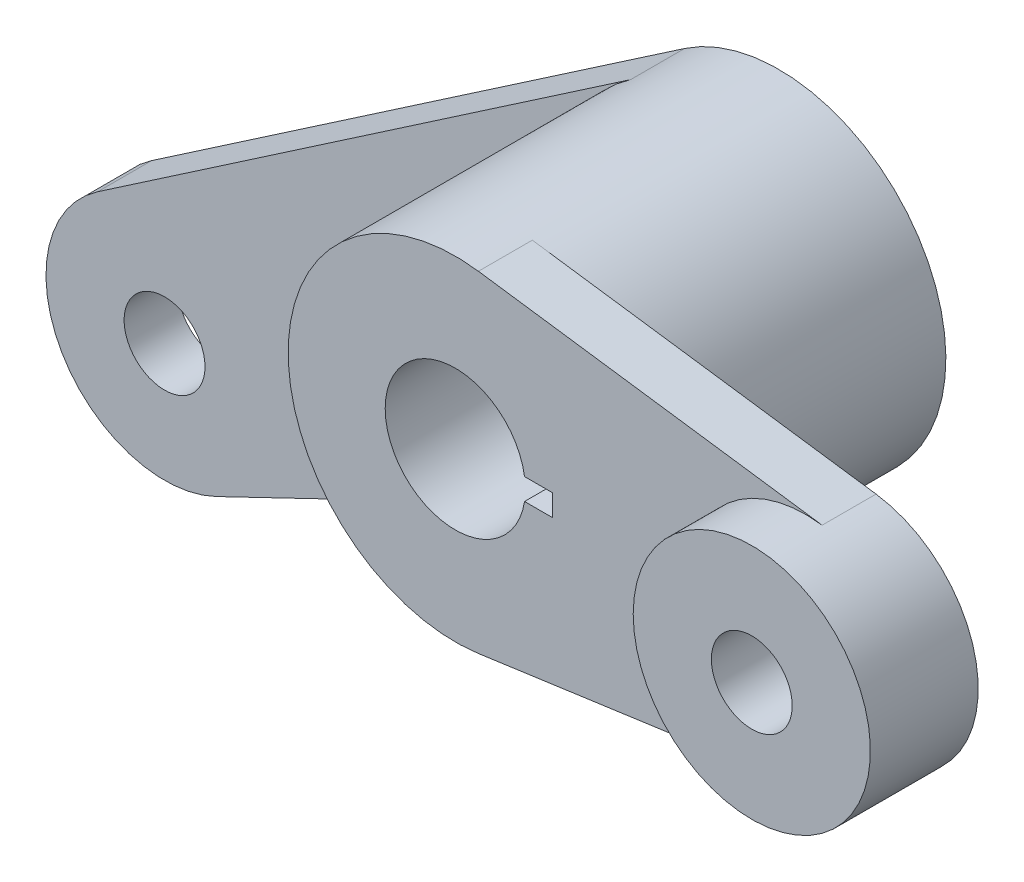
ISO-10303-21;
HEADER;
FILE_DESCRIPTION(('STEP AP214'),'2;1');
FILE_NAME('part.step','',(''),(''),'','','');
FILE_SCHEMA(('AUTOMOTIVE_DESIGN { 1 0 10303 214 1 1 1 1 }'));
ENDSEC;
DATA;
#1=APPLICATION_CONTEXT('core data for automotive mechanical design processes');
#2=APPLICATION_PROTOCOL_DEFINITION('international standard','automotive_design',2000,#1);
#3=PRODUCT_CONTEXT('',#1,'mechanical');
#4=PRODUCT('Part','Part','',(#3));
#5=PRODUCT_RELATED_PRODUCT_CATEGORY('part','',(#4));
#6=PRODUCT_DEFINITION_FORMATION('','',#4);
#7=PRODUCT_DEFINITION_CONTEXT('part definition',#1,'design');
#8=PRODUCT_DEFINITION('design','',#6,#7);
#9=PRODUCT_DEFINITION_SHAPE('','',#8);
#10=(LENGTH_UNIT() NAMED_UNIT(*) SI_UNIT(.MILLI.,.METRE.));
#11=(NAMED_UNIT(*) PLANE_ANGLE_UNIT() SI_UNIT($,.RADIAN.));
#12=(NAMED_UNIT(*) SI_UNIT($,.STERADIAN.) SOLID_ANGLE_UNIT());
#13=UNCERTAINTY_MEASURE_WITH_UNIT(LENGTH_MEASURE(1.E-05),#10,'distance_accuracy_value','');
#14=(GEOMETRIC_REPRESENTATION_CONTEXT(3) GLOBAL_UNCERTAINTY_ASSIGNED_CONTEXT((#13)) GLOBAL_UNIT_ASSIGNED_CONTEXT((#10,
#11,#12)) REPRESENTATION_CONTEXT('',''));
#15=CARTESIAN_POINT('',(0.,0.,0.));
#16=DIRECTION('',(0.,0.,1.));
#17=DIRECTION('',(1.,0.,0.));
#18=AXIS2_PLACEMENT_3D('',#15,#16,#17);
#19=CARTESIAN_POINT('',(65.,0.,-10.));
#20=DIRECTION('',(0.,0.,1.));
#21=DIRECTION('',(1.,0.,0.));
#22=AXIS2_PLACEMENT_3D('',#19,#20,#21);
#23=PLANE('',#22);
#24=CARTESIAN_POINT('',(65.,0.,-10.000012));
#25=DIRECTION('',(0.,0.,-1.));
#26=DIRECTION('',(-1.,0.,0.));
#27=AXIS2_PLACEMENT_3D('',#24,#25,#26);
#28=CIRCLE('',#27,7.5);
#29=CARTESIAN_POINT('',(57.5,0.,-10.000012));
#30=VERTEX_POINT('',#29);
#31=EDGE_CURVE('E198',#30,#30,#28,.T.);
#32=ORIENTED_EDGE('',*,*,#31,.F.);
#33=EDGE_LOOP('',(#32));
#34=FACE_BOUND('',#33,.T.);
#35=CARTESIAN_POINT('',(0.,0.,-10.));
#36=DIRECTION('',(0.,0.,-1.));
#37=DIRECTION('',(-1.,0.,0.));
#38=AXIS2_PLACEMENT_3D('',#35,#36,#37);
#39=CIRCLE('',#38,31.);
#40=CARTESIAN_POINT('',(4.29230769230769,30.7014021613762,-10.));
#41=VERTEX_POINT('',#40);
#42=CARTESIAN_POINT('',(4.29230769230769,-30.7014021613762,-10.));
#43=VERTEX_POINT('',#42);
#44=EDGE_CURVE('E193',#41,#43,#39,.T.);
#45=ORIENTED_EDGE('',*,*,#44,.F.);
#46=DIRECTION('',(-0.990367811657297,0.138461538461539,0.));
#47=VECTOR('',#46,1.);
#48=CARTESIAN_POINT('',(4.29230769230769,30.7014021613762,-10.));
#49=LINE('',#48,#47);
#50=CARTESIAN_POINT('',(68.0461538461538,21.7880918564605,-10.));
#51=VERTEX_POINT('',#50);
#52=EDGE_CURVE('E208',#51,#41,#49,.T.);
#53=ORIENTED_EDGE('',*,*,#52,.F.);
#54=CARTESIAN_POINT('',(65.,0.,-10.));
#55=DIRECTION('',(0.,0.,1.));
#56=DIRECTION('',(1.,0.,0.));
#57=AXIS2_PLACEMENT_3D('',#54,#55,#56);
#58=CIRCLE('',#57,22.);
#59=CARTESIAN_POINT('',(68.0461538461539,-21.7880918564605,-10.));
#60=VERTEX_POINT('',#59);
#61=EDGE_CURVE('E202',#60,#51,#58,.T.);
#62=ORIENTED_EDGE('',*,*,#61,.F.);
#63=DIRECTION('',(0.990367811657297,0.138461538461538,0.));
#64=VECTOR('',#63,1.);
#65=CARTESIAN_POINT('',(68.0461538461539,-21.7880918564605,-10.));
#66=LINE('',#65,#64);
#67=EDGE_CURVE('E215',#43,#60,#66,.T.);
#68=ORIENTED_EDGE('',*,*,#67,.F.);
#69=EDGE_LOOP('',(#45,#53,#62,#68));
#70=FACE_BOUND('',#69,.T.);
#71=ADVANCED_FACE('F39',(#34,#70),#23,.F.);
#72=CARTESIAN_POINT('',(65.,0.,-10.));
#73=DIRECTION('',(0.,0.,1.));
#74=DIRECTION('',(1.,0.,0.));
#75=AXIS2_PLACEMENT_3D('',#72,#73,#74);
#76=CYLINDRICAL_SURFACE('',#75,22.);
#77=DIRECTION('',(0.,0.,1.));
#78=VECTOR('',#77,1.);
#79=CARTESIAN_POINT('',(68.0461538461538,21.7880918564605,-10.));
#80=LINE('',#79,#78);
#81=CARTESIAN_POINT('',(68.0461538461538,21.7880918564605,0.));
#82=VERTEX_POINT('',#81);
#83=EDGE_CURVE('E214',#51,#82,#80,.T.);
#84=ORIENTED_EDGE('',*,*,#83,.T.);
#85=CARTESIAN_POINT('',(65.,0.,0.));
#86=DIRECTION('',(0.,0.,1.));
#87=DIRECTION('',(1.,0.,0.));
#88=AXIS2_PLACEMENT_3D('',#85,#86,#87);
#89=CIRCLE('',#88,22.);
#90=CARTESIAN_POINT('',(68.0461538461539,-21.7880918564605,0.));
#91=VERTEX_POINT('',#90);
#92=EDGE_CURVE('E223',#82,#91,#89,.T.);
#93=ORIENTED_EDGE('',*,*,#92,.T.);
#94=DIRECTION('',(0.,0.,1.));
#95=VECTOR('',#94,1.);
#96=CARTESIAN_POINT('',(68.0461538461539,-21.7880918564605,-10.));
#97=LINE('',#96,#95);
#98=EDGE_CURVE('E224',#60,#91,#97,.T.);
#99=ORIENTED_EDGE('',*,*,#98,.F.);
#100=ORIENTED_EDGE('',*,*,#61,.T.);
#101=EDGE_LOOP('',(#84,#93,#99,#100));
#102=FACE_BOUND('',#101,.T.);
#103=CARTESIAN_POINT('',(65.,0.,10.));
#104=DIRECTION('',(0.,0.,-1.));
#105=DIRECTION('',(-1.,0.,0.));
#106=AXIS2_PLACEMENT_3D('',#103,#104,#105);
#107=CIRCLE('',#106,22.);
#108=CARTESIAN_POINT('',(43.,0.,10.));
#109=VERTEX_POINT('',#108);
#110=EDGE_CURVE('E203',#109,#109,#107,.T.);
#111=ORIENTED_EDGE('',*,*,#110,.T.);
#112=EDGE_LOOP('',(#111));
#113=FACE_BOUND('',#112,.T.);
#114=ADVANCED_FACE('F41',(#102,#113),#76,.T.);
#115=CARTESIAN_POINT('',(68.0461538461539,-21.7880918564605,-10.));
#116=DIRECTION('',(0.138461538461538,-0.990367811657297,0.));
#117=DIRECTION('',(0.990367811657297,0.138461538461538,0.));
#118=AXIS2_PLACEMENT_3D('',#115,#116,#117);
#119=PLANE('',#118);
#120=DIRECTION('',(0.990367811657297,0.138461538461538,0.));
#121=VECTOR('',#120,1.);
#122=CARTESIAN_POINT('',(68.0461538461539,-21.7880918564605,0.));
#123=LINE('',#122,#121);
#124=CARTESIAN_POINT('',(4.29230769230769,-30.7014021613762,0.));
#125=VERTEX_POINT('',#124);
#126=EDGE_CURVE('E207',#125,#91,#123,.T.);
#127=ORIENTED_EDGE('',*,*,#126,.F.);
#128=DIRECTION('',(0.,0.,1.));
#129=VECTOR('',#128,1.);
#130=CARTESIAN_POINT('',(4.29230769230769,-30.7014021613762,-10.));
#131=LINE('',#130,#129);
#132=EDGE_CURVE('E228',#43,#125,#131,.T.);
#133=ORIENTED_EDGE('',*,*,#132,.F.);
#134=ORIENTED_EDGE('',*,*,#67,.T.);
#135=ORIENTED_EDGE('',*,*,#98,.T.);
#136=EDGE_LOOP('',(#127,#133,#134,#135));
#137=FACE_BOUND('',#136,.T.);
#138=ADVANCED_FACE('F259',(#137),#119,.T.);
#139=CARTESIAN_POINT('',(0.,0.,-10.));
#140=DIRECTION('',(0.,0.,1.));
#141=DIRECTION('',(1.,0.,0.));
#142=AXIS2_PLACEMENT_3D('',#139,#140,#141);
#143=CYLINDRICAL_SURFACE('',#142,31.);
#144=CARTESIAN_POINT('',(0.,0.,0.));
#145=DIRECTION('',(0.,0.,1.));
#146=DIRECTION('',(1.,0.,0.));
#147=AXIS2_PLACEMENT_3D('',#144,#145,#146);
#148=CIRCLE('',#147,31.);
#149=CARTESIAN_POINT('',(4.29230769230769,30.7014021613762,0.));
#150=VERTEX_POINT('',#149);
#151=EDGE_CURVE('E217',#150,#125,#148,.T.);
#152=ORIENTED_EDGE('',*,*,#151,.F.);
#153=DIRECTION('',(0.,0.,1.));
#154=VECTOR('',#153,1.);
#155=CARTESIAN_POINT('',(4.29230769230769,30.7014021613762,-10.));
#156=LINE('',#155,#154);
#157=EDGE_CURVE('E226',#41,#150,#156,.T.);
#158=ORIENTED_EDGE('',*,*,#157,.F.);
#159=ORIENTED_EDGE('',*,*,#44,.T.);
#160=ORIENTED_EDGE('',*,*,#132,.T.);
#161=EDGE_LOOP('',(#152,#158,#159,#160));
#162=FACE_BOUND('',#161,.T.);
#163=CARTESIAN_POINT('',(0.,0.,-50.));
#164=DIRECTION('',(0.,0.,-1.));
#165=DIRECTION('',(-1.,0.,0.));
#166=AXIS2_PLACEMENT_3D('',#163,#164,#165);
#167=CIRCLE('',#166,31.);
#168=CARTESIAN_POINT('',(13.442835709465,-27.9336744465946,-50.));
#169=VERTEX_POINT('',#168);
#170=CARTESIAN_POINT('',(-17.4698538370627,25.6086744465946,-50.));
#171=VERTEX_POINT('',#170);
#172=EDGE_CURVE('E53',#169,#171,#167,.T.);
#173=ORIENTED_EDGE('',*,*,#172,.F.);
#174=DIRECTION('',(0.,0.,1.));
#175=VECTOR('',#174,1.);
#176=CARTESIAN_POINT('',(13.442835709465,-27.9336744465946,-60.));
#177=LINE('',#176,#175);
#178=CARTESIAN_POINT('',(13.442835709465,-27.9336744465946,-60.));
#179=VERTEX_POINT('',#178);
#180=EDGE_CURVE('E182',#179,#169,#177,.T.);
#181=ORIENTED_EDGE('',*,*,#180,.F.);
#182=CARTESIAN_POINT('',(0.,0.,-60.));
#183=DIRECTION('',(0.,0.,1.));
#184=DIRECTION('',(1.,0.,0.));
#185=AXIS2_PLACEMENT_3D('',#182,#183,#184);
#186=CIRCLE('',#185,31.);
#187=CARTESIAN_POINT('',(-17.4698538370627,25.6086744465946,-60.));
#188=VERTEX_POINT('',#187);
#189=EDGE_CURVE('E159',#179,#188,#186,.T.);
#190=ORIENTED_EDGE('',*,*,#189,.T.);
#191=DIRECTION('',(0.,0.,1.));
#192=VECTOR('',#191,1.);
#193=CARTESIAN_POINT('',(-17.4698538370627,25.6086744465946,-60.));
#194=LINE('',#193,#192);
#195=EDGE_CURVE('E171',#188,#171,#194,.T.);
#196=ORIENTED_EDGE('',*,*,#195,.T.);
#197=EDGE_LOOP('',(#173,#181,#190,#196));
#198=FACE_BOUND('',#197,.T.);
#199=ADVANCED_FACE('F265',(#162,#198),#143,.T.);
#200=CARTESIAN_POINT('',(4.29230769230769,30.7014021613762,-10.));
#201=DIRECTION('',(0.138461538461539,0.990367811657297,0.));
#202=DIRECTION('',(-0.990367811657297,0.138461538461539,0.));
#203=AXIS2_PLACEMENT_3D('',#200,#201,#202);
#204=PLANE('',#203);
#205=DIRECTION('',(-0.990367811657297,0.138461538461539,0.));
#206=VECTOR('',#205,1.);
#207=CARTESIAN_POINT('',(4.29230769230769,30.7014021613762,0.));
#208=LINE('',#207,#206);
#209=EDGE_CURVE('E204',#82,#150,#208,.T.);
#210=ORIENTED_EDGE('',*,*,#209,.F.);
#211=ORIENTED_EDGE('',*,*,#83,.F.);
#212=ORIENTED_EDGE('',*,*,#52,.T.);
#213=ORIENTED_EDGE('',*,*,#157,.T.);
#214=EDGE_LOOP('',(#210,#211,#212,#213));
#215=FACE_BOUND('',#214,.T.);
#216=ADVANCED_FACE('F260',(#215),#204,.T.);
#217=CARTESIAN_POINT('',(65.,0.,0.));
#218=DIRECTION('',(0.,0.,1.));
#219=DIRECTION('',(1.,0.,0.));
#220=AXIS2_PLACEMENT_3D('',#217,#218,#219);
#221=PLANE('',#220);
#222=DIRECTION('',(0.,1.,0.));
#223=VECTOR('',#222,1.);
#224=CARTESIAN_POINT('',(18.,0.,0.));
#225=LINE('',#224,#223);
#226=CARTESIAN_POINT('',(18.,-2.,0.));
#227=VERTEX_POINT('',#226);
#228=CARTESIAN_POINT('',(18.,2.,0.));
#229=VERTEX_POINT('',#228);
#230=EDGE_CURVE('E11',#227,#229,#225,.T.);
#231=ORIENTED_EDGE('',*,*,#230,.F.);
#232=DIRECTION('',(1.,0.,0.));
#233=VECTOR('',#232,1.);
#234=CARTESIAN_POINT('',(65.,-1.99999999999997,0.));
#235=LINE('',#234,#233);
#236=CARTESIAN_POINT('',(12.8452325786651,-2.,0.));
#237=VERTEX_POINT('',#236);
#238=EDGE_CURVE('E131',#237,#227,#235,.T.);
#239=ORIENTED_EDGE('',*,*,#238,.F.);
#240=CARTESIAN_POINT('',(0.,0.,0.));
#241=DIRECTION('',(0.,0.,1.));
#242=DIRECTION('',(1.,0.,0.));
#243=AXIS2_PLACEMENT_3D('',#240,#241,#242);
#244=CIRCLE('',#243,13.);
#245=CARTESIAN_POINT('',(12.8452325786651,2.,0.));
#246=VERTEX_POINT('',#245);
#247=EDGE_CURVE('E181',#246,#237,#244,.T.);
#248=ORIENTED_EDGE('',*,*,#247,.F.);
#249=DIRECTION('',(-1.,0.,0.));
#250=VECTOR('',#249,1.);
#251=CARTESIAN_POINT('',(65.,1.99999999999998,0.));
#252=LINE('',#251,#250);
#253=EDGE_CURVE('E50',#229,#246,#252,.T.);
#254=ORIENTED_EDGE('',*,*,#253,.F.);
#255=EDGE_LOOP('',(#231,#239,#248,#254));
#256=FACE_BOUND('',#255,.T.);
#257=ORIENTED_EDGE('',*,*,#92,.F.);
#258=ORIENTED_EDGE('',*,*,#209,.T.);
#259=ORIENTED_EDGE('',*,*,#151,.T.);
#260=ORIENTED_EDGE('',*,*,#126,.T.);
#261=EDGE_LOOP('',(#257,#258,#259,#260));
#262=FACE_BOUND('',#261,.T.);
#263=ADVANCED_FACE('F255',(#256,#262),#221,.T.);
#264=CARTESIAN_POINT('',(65.,0.,10.));
#265=DIRECTION('',(0.,0.,-1.));
#266=DIRECTION('',(-1.,0.,0.));
#267=AXIS2_PLACEMENT_3D('',#264,#265,#266);
#268=PLANE('',#267);
#269=CARTESIAN_POINT('',(65.,0.,10.));
#270=DIRECTION('',(0.,0.,-1.));
#271=DIRECTION('',(-1.,0.,0.));
#272=AXIS2_PLACEMENT_3D('',#269,#270,#271);
#273=CIRCLE('',#272,7.5);
#274=CARTESIAN_POINT('',(57.5,0.,10.));
#275=VERTEX_POINT('',#274);
#276=EDGE_CURVE('E196',#275,#275,#273,.T.);
#277=ORIENTED_EDGE('',*,*,#276,.T.);
#278=EDGE_LOOP('',(#277));
#279=FACE_BOUND('',#278,.T.);
#280=ORIENTED_EDGE('',*,*,#110,.F.);
#281=EDGE_LOOP('',(#280));
#282=FACE_BOUND('',#281,.T.);
#283=ADVANCED_FACE('F252',(#279,#282),#268,.F.);
#284=CARTESIAN_POINT('',(65.,0.,10.));
#285=DIRECTION('',(0.,0.,-1.));
#286=DIRECTION('',(-1.,0.,0.));
#287=AXIS2_PLACEMENT_3D('',#284,#285,#286);
#288=CYLINDRICAL_SURFACE('',#287,7.5);
#289=ORIENTED_EDGE('',*,*,#276,.F.);
#290=EDGE_LOOP('',(#289));
#291=FACE_BOUND('',#290,.T.);
#292=ORIENTED_EDGE('',*,*,#31,.T.);
#293=EDGE_LOOP('',(#292));
#294=FACE_BOUND('',#293,.T.);
#295=ADVANCED_FACE('F286',(#291,#294),#288,.F.);
#296=CARTESIAN_POINT('',(0.,0.,-50.));
#297=DIRECTION('',(0.,0.,1.));
#298=DIRECTION('',(1.,0.,0.));
#299=AXIS2_PLACEMENT_3D('',#296,#297,#298);
#300=CYLINDRICAL_SURFACE('',#299,13.);
#301=DIRECTION('',(0.,0.,1.));
#302=VECTOR('',#301,1.);
#303=CARTESIAN_POINT('',(12.8452325786651,2.,-50.));
#304=LINE('',#303,#302);
#305=CARTESIAN_POINT('',(12.8452325786651,2.,-60.));
#306=VERTEX_POINT('',#305);
#307=EDGE_CURVE('E195',#306,#246,#304,.T.);
#308=ORIENTED_EDGE('',*,*,#307,.T.);
#309=ORIENTED_EDGE('',*,*,#247,.T.);
#310=DIRECTION('',(0.,0.,1.));
#311=VECTOR('',#310,1.);
#312=CARTESIAN_POINT('',(12.8452325786651,-2.,-50.));
#313=LINE('',#312,#311);
#314=CARTESIAN_POINT('',(12.8452325786651,-2.,-60.));
#315=VERTEX_POINT('',#314);
#316=EDGE_CURVE('E65',#315,#237,#313,.T.);
#317=ORIENTED_EDGE('',*,*,#316,.F.);
#318=CARTESIAN_POINT('',(0.,0.,-60.));
#319=DIRECTION('',(0.,0.,1.));
#320=DIRECTION('',(1.,0.,0.));
#321=AXIS2_PLACEMENT_3D('',#318,#319,#320);
#322=CIRCLE('',#321,13.);
#323=EDGE_CURVE('E149',#306,#315,#322,.T.);
#324=ORIENTED_EDGE('',*,*,#323,.F.);
#325=EDGE_LOOP('',(#308,#309,#317,#324));
#326=FACE_BOUND('',#325,.T.);
#327=ADVANCED_FACE('F292',(#326),#300,.F.);
#328=CARTESIAN_POINT('',(12.8452325786651,2.,-50.));
#329=DIRECTION('',(0.,-1.,0.));
#330=DIRECTION('',(0.,0.,-1.));
#331=AXIS2_PLACEMENT_3D('',#328,#329,#330);
#332=PLANE('',#331);
#333=DIRECTION('',(0.,0.,1.));
#334=VECTOR('',#333,1.);
#335=CARTESIAN_POINT('',(18.,2.,-50.));
#336=LINE('',#335,#334);
#337=CARTESIAN_POINT('',(18.,2.,-60.));
#338=VERTEX_POINT('',#337);
#339=EDGE_CURVE('E136',#338,#229,#336,.T.);
#340=ORIENTED_EDGE('',*,*,#339,.T.);
#341=ORIENTED_EDGE('',*,*,#253,.T.);
#342=ORIENTED_EDGE('',*,*,#307,.F.);
#343=DIRECTION('',(-1.,0.,0.));
#344=VECTOR('',#343,1.);
#345=CARTESIAN_POINT('',(18.,2.,-60.));
#346=LINE('',#345,#344);
#347=EDGE_CURVE('E145',#338,#306,#346,.T.);
#348=ORIENTED_EDGE('',*,*,#347,.F.);
#349=EDGE_LOOP('',(#340,#341,#342,#348));
#350=FACE_BOUND('',#349,.T.);
#351=ADVANCED_FACE('F296',(#350),#332,.T.);
#352=CARTESIAN_POINT('',(18.,-2.,-50.));
#353=DIRECTION('',(-1.,0.,0.));
#354=DIRECTION('',(0.,0.,1.));
#355=AXIS2_PLACEMENT_3D('',#352,#353,#354);
#356=PLANE('',#355);
#357=DIRECTION('',(0.,0.,1.));
#358=VECTOR('',#357,1.);
#359=CARTESIAN_POINT('',(18.,-2.,-50.));
#360=LINE('',#359,#358);
#361=CARTESIAN_POINT('',(18.,-2.,-60.));
#362=VERTEX_POINT('',#361);
#363=EDGE_CURVE('E127',#362,#227,#360,.T.);
#364=ORIENTED_EDGE('',*,*,#363,.T.);
#365=ORIENTED_EDGE('',*,*,#230,.T.);
#366=ORIENTED_EDGE('',*,*,#339,.F.);
#367=DIRECTION('',(0.,1.,0.));
#368=VECTOR('',#367,1.);
#369=CARTESIAN_POINT('',(18.,-2.,-60.));
#370=LINE('',#369,#368);
#371=EDGE_CURVE('E138',#362,#338,#370,.T.);
#372=ORIENTED_EDGE('',*,*,#371,.F.);
#373=EDGE_LOOP('',(#364,#365,#366,#372));
#374=FACE_BOUND('',#373,.T.);
#375=ADVANCED_FACE('F139',(#374),#356,.T.);
#376=CARTESIAN_POINT('',(12.8452325786651,-2.,-50.));
#377=DIRECTION('',(0.,1.,0.));
#378=DIRECTION('',(-1.,0.,0.));
#379=AXIS2_PLACEMENT_3D('',#376,#377,#378);
#380=PLANE('',#379);
#381=ORIENTED_EDGE('',*,*,#316,.T.);
#382=ORIENTED_EDGE('',*,*,#238,.T.);
#383=ORIENTED_EDGE('',*,*,#363,.F.);
#384=DIRECTION('',(1.,0.,0.));
#385=VECTOR('',#384,1.);
#386=CARTESIAN_POINT('',(12.8452325786651,-2.,-60.));
#387=LINE('',#386,#385);
#388=EDGE_CURVE('E128',#315,#362,#387,.T.);
#389=ORIENTED_EDGE('',*,*,#388,.F.);
#390=EDGE_LOOP('',(#381,#382,#383,#389));
#391=FACE_BOUND('',#390,.T.);
#392=ADVANCED_FACE('F126',(#391),#380,.T.);
#393=CARTESIAN_POINT('',(-94.3829714990283,-79.8238979943576,-60.));
#394=DIRECTION('',(0.433639861595647,-0.901086272470793,0.));
#395=DIRECTION('',(0.901086272470793,0.433639861595647,0.));
#396=AXIS2_PLACEMENT_3D('',#393,#394,#395);
#397=PLANE('',#396);
#398=DIRECTION('',(0.901086272470793,0.433639861595647,0.));
#399=VECTOR('',#398,1.);
#400=CARTESIAN_POINT('',(-94.3829714990283,-79.8238979943576,-50.));
#401=LINE('',#400,#399);
#402=CARTESIAN_POINT('',(-94.3829714990283,-79.8238979943576,-50.));
#403=VERTEX_POINT('',#402);
#404=EDGE_CURVE('E163',#403,#169,#401,.T.);
#405=ORIENTED_EDGE('',*,*,#404,.F.);
#406=DIRECTION('',(0.,0.,1.));
#407=VECTOR('',#406,1.);
#408=CARTESIAN_POINT('',(-94.3829714990283,-79.8238979943576,-60.));
#409=LINE('',#408,#407);
#410=CARTESIAN_POINT('',(-94.3829714990283,-79.8238979943576,-60.));
#411=VERTEX_POINT('',#410);
#412=EDGE_CURVE('E184',#411,#403,#409,.T.);
#413=ORIENTED_EDGE('',*,*,#412,.F.);
#414=DIRECTION('',(0.901086272470793,0.433639861595647,0.));
#415=VECTOR('',#414,1.);
#416=CARTESIAN_POINT('',(-94.3829714990283,-79.8238979943576,-60.));
#417=LINE('',#416,#415);
#418=EDGE_CURVE('E168',#411,#179,#417,.T.);
#419=ORIENTED_EDGE('',*,*,#418,.T.);
#420=ORIENTED_EDGE('',*,*,#180,.T.);
#421=EDGE_LOOP('',(#405,#413,#419,#420));
#422=FACE_BOUND('',#421,.T.);
#423=ADVANCED_FACE('F323',(#422),#397,.T.);
#424=CARTESIAN_POINT('',(-103.923048454133,-60.0000000000002,-60.));
#425=DIRECTION('',(0.,0.,1.));
#426=DIRECTION('',(1.,0.,0.));
#427=AXIS2_PLACEMENT_3D('',#424,#425,#426);
#428=CYLINDRICAL_SURFACE('',#427,22.);
#429=CARTESIAN_POINT('',(-103.923048454133,-60.0000000000002,-50.));
#430=DIRECTION('',(0.,0.,1.));
#431=DIRECTION('',(1.,0.,0.));
#432=AXIS2_PLACEMENT_3D('',#429,#430,#431);
#433=CIRCLE('',#432,22.);
#434=CARTESIAN_POINT('',(-116.321009241725,-41.8261020056427,-50.));
#435=VERTEX_POINT('',#434);
#436=EDGE_CURVE('E176',#435,#403,#433,.T.);
#437=ORIENTED_EDGE('',*,*,#436,.F.);
#438=DIRECTION('',(0.,0.,1.));
#439=VECTOR('',#438,1.);
#440=CARTESIAN_POINT('',(-116.321009241725,-41.8261020056427,-60.));
#441=LINE('',#440,#439);
#442=CARTESIAN_POINT('',(-116.321009241725,-41.8261020056427,-60.));
#443=VERTEX_POINT('',#442);
#444=EDGE_CURVE('E188',#443,#435,#441,.T.);
#445=ORIENTED_EDGE('',*,*,#444,.F.);
#446=CARTESIAN_POINT('',(-103.923048454133,-60.0000000000002,-60.));
#447=DIRECTION('',(0.,0.,1.));
#448=DIRECTION('',(1.,0.,0.));
#449=AXIS2_PLACEMENT_3D('',#446,#447,#448);
#450=CIRCLE('',#449,22.);
#451=EDGE_CURVE('E170',#443,#411,#450,.T.);
#452=ORIENTED_EDGE('',*,*,#451,.T.);
#453=ORIENTED_EDGE('',*,*,#412,.T.);
#454=EDGE_LOOP('',(#437,#445,#452,#453));
#455=FACE_BOUND('',#454,.T.);
#456=ADVANCED_FACE('F330',(#455),#428,.T.);
#457=CARTESIAN_POINT('',(-17.4698538370627,25.6086744465946,-60.));
#458=DIRECTION('',(-0.563543672163313,0.826086272470793,0.));
#459=DIRECTION('',(-0.826086272470793,-0.563543672163313,0.));
#460=AXIS2_PLACEMENT_3D('',#457,#458,#459);
#461=PLANE('',#460);
#462=DIRECTION('',(-0.826086272470793,-0.563543672163312,0.));
#463=VECTOR('',#462,1.);
#464=CARTESIAN_POINT('',(-17.4698538370627,25.6086744465946,-50.));
#465=LINE('',#464,#463);
#466=EDGE_CURVE('E157',#171,#435,#465,.T.);
#467=ORIENTED_EDGE('',*,*,#466,.F.);
#468=ORIENTED_EDGE('',*,*,#195,.F.);
#469=DIRECTION('',(-0.826086272470793,-0.563543672163312,0.));
#470=VECTOR('',#469,1.);
#471=CARTESIAN_POINT('',(-17.4698538370627,25.6086744465946,-60.));
#472=LINE('',#471,#470);
#473=EDGE_CURVE('E162',#188,#443,#472,.T.);
#474=ORIENTED_EDGE('',*,*,#473,.T.);
#475=ORIENTED_EDGE('',*,*,#444,.T.);
#476=EDGE_LOOP('',(#467,#468,#474,#475));
#477=FACE_BOUND('',#476,.T.);
#478=ADVANCED_FACE('F322',(#477),#461,.T.);
#479=CARTESIAN_POINT('',(0.,0.,-60.));
#480=DIRECTION('',(0.,0.,1.));
#481=DIRECTION('',(1.,0.,0.));
#482=AXIS2_PLACEMENT_3D('',#479,#480,#481);
#483=PLANE('',#482);
#484=CARTESIAN_POINT('',(-103.923048454133,-60.0000000000002,-60.));
#485=DIRECTION('',(0.,0.,1.));
#486=DIRECTION('',(1.,0.,0.));
#487=AXIS2_PLACEMENT_3D('',#484,#485,#486);
#488=CIRCLE('',#487,7.5);
#489=CARTESIAN_POINT('',(-96.4230484541326,-60.0000000000002,-60.));
#490=VERTEX_POINT('',#489);
#491=EDGE_CURVE('E147',#490,#490,#488,.T.);
#492=ORIENTED_EDGE('',*,*,#491,.T.);
#493=EDGE_LOOP('',(#492));
#494=FACE_BOUND('',#493,.T.);
#495=ORIENTED_EDGE('',*,*,#323,.T.);
#496=ORIENTED_EDGE('',*,*,#388,.T.);
#497=ORIENTED_EDGE('',*,*,#371,.T.);
#498=ORIENTED_EDGE('',*,*,#347,.T.);
#499=EDGE_LOOP('',(#495,#496,#497,#498));
#500=FACE_BOUND('',#499,.T.);
#501=ORIENTED_EDGE('',*,*,#189,.F.);
#502=ORIENTED_EDGE('',*,*,#418,.F.);
#503=ORIENTED_EDGE('',*,*,#451,.F.);
#504=ORIENTED_EDGE('',*,*,#473,.F.);
#505=EDGE_LOOP('',(#501,#502,#503,#504));
#506=FACE_BOUND('',#505,.T.);
#507=ADVANCED_FACE('F148',(#494,#500,#506),#483,.F.);
#508=CARTESIAN_POINT('',(0.,0.,-50.));
#509=DIRECTION('',(0.,0.,1.));
#510=DIRECTION('',(1.,0.,0.));
#511=AXIS2_PLACEMENT_3D('',#508,#509,#510);
#512=PLANE('',#511);
#513=CARTESIAN_POINT('',(-103.923048454133,-60.0000000000002,-50.));
#514=DIRECTION('',(0.,0.,1.));
#515=DIRECTION('',(1.,0.,0.));
#516=AXIS2_PLACEMENT_3D('',#513,#514,#515);
#517=CIRCLE('',#516,7.5);
#518=CARTESIAN_POINT('',(-96.4230484541326,-60.0000000000002,-50.));
#519=VERTEX_POINT('',#518);
#520=EDGE_CURVE('E153',#519,#519,#517,.T.);
#521=ORIENTED_EDGE('',*,*,#520,.F.);
#522=EDGE_LOOP('',(#521));
#523=FACE_BOUND('',#522,.T.);
#524=ORIENTED_EDGE('',*,*,#404,.T.);
#525=ORIENTED_EDGE('',*,*,#172,.T.);
#526=ORIENTED_EDGE('',*,*,#466,.T.);
#527=ORIENTED_EDGE('',*,*,#436,.T.);
#528=EDGE_LOOP('',(#524,#525,#526,#527));
#529=FACE_BOUND('',#528,.T.);
#530=ADVANCED_FACE('F333',(#523,#529),#512,.T.);
#531=CARTESIAN_POINT('',(-103.923048454133,-60.0000000000002,-60.));
#532=DIRECTION('',(0.,0.,1.));
#533=DIRECTION('',(1.,0.,0.));
#534=AXIS2_PLACEMENT_3D('',#531,#532,#533);
#535=CYLINDRICAL_SURFACE('',#534,7.5);
#536=ORIENTED_EDGE('',*,*,#491,.F.);
#537=EDGE_LOOP('',(#536));
#538=FACE_BOUND('',#537,.T.);
#539=ORIENTED_EDGE('',*,*,#520,.T.);
#540=EDGE_LOOP('',(#539));
#541=FACE_BOUND('',#540,.T.);
#542=ADVANCED_FACE('F336',(#538,#541),#535,.F.);
#543=CLOSED_SHELL('',(#71,#114,#138,#199,#216,#263,#283,#295,#327,#351,#375,#392,#423,#456,#478,
#507,#530,#542));
#544=MANIFOLD_SOLID_BREP('B2',#543);
#545=ADVANCED_BREP_SHAPE_REPRESENTATION('',(#18,#544),#14);
#546=SHAPE_DEFINITION_REPRESENTATION(#9,#545);
ENDSEC;
END-ISO-10303-21;
